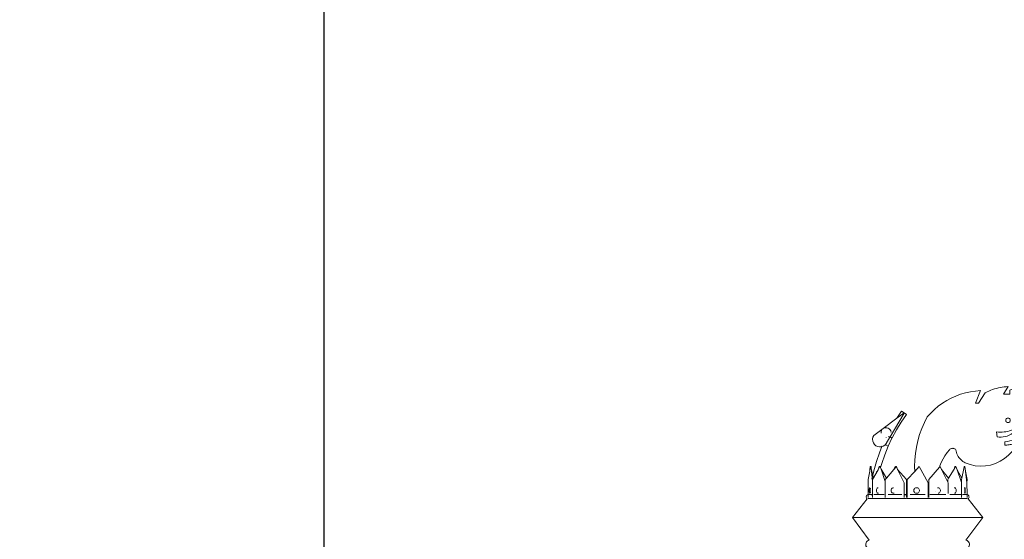
# Model space of a CAD drawing. Units: millimetres. Extents: x 7894 to 8038, y 6851 to 6951.
# Tile 22 of 49: x 7946.6 to 7958.7, y 6910.05 to 6916.43. Entities that reach past the tile are written whole.
import ezdxf

# ---------------------------------------------------------------- set-up
doc = ezdxf.new("R2010")
doc.units = ezdxf.units.MM
doc.layers.add('A-ANNO-DIMS', color=2, linetype='Continuous', lineweight=18)
doc.layers.add('A-FURN-ACCS', color=8, linetype='Continuous', lineweight=13)
doc.styles.get("Standard").update_dxf_attribs({"font": 'arial.ttf'})
doc.dimstyles.new('ISO-25', dxfattribs={"dimtxt": 1, "dimasz": 1, "dimexe": 1.25, "dimexo": 0.625, "dimtad": 1, "dimdec": 0, "dimlunit": 4, "dimtxsty": 'Standard', "dimcen": 2.5, "dimclrt": 1, "dimadec": 0, "dimazin": 0, "dimtfac": 1, "dimtdec": 0, "dimtmove": 0, "dimatfit": 3, "dimfxl": 1, "dimarcsym": 0})

# ---------------------------------------------------------------- blocks, each defined once
blk = doc.blocks.new('DISPLAY-LEAF-FINIAL')
for p, q in [((2.565, 3.508), (2.565, 3.494)), ((2.209, 3.334), (2.276, 3.441)), ((2.276, 3.441), (2.398, 3.441)), ((2.398, 3.441), (2.409, 3.452)), ((2.409, 3.452), (2.421, 3.461)), ((2.421, 3.461), (2.434, 3.47)), ((2.434, 3.47), (2.447, 3.478)), ((2.447, 3.478), (2.461, 3.485)), ((2.461, 3.485), (2.475, 3.491)), ((2.475, 3.491), (2.489, 3.496)), ((2.489, 3.496), (2.504, 3.501)), ((2.504, 3.501), (2.519, 3.504)), ((2.516, 3.389), (2.505, 3.379)), ((2.527, 3.4), (2.516, 3.389)), ((2.536, 3.411), (2.527, 3.4)), ((2.544, 3.424), (2.536, 3.411)), ((2.551, 3.437), (2.544, 3.424)), ((2.556, 3.45), (2.551, 3.437)), ((2.56, 3.465), (2.556, 3.45)), ((2.563, 3.479), (2.56, 3.465)), ((2.565, 3.494), (2.563, 3.479)), ((2.023, 3.221), (2.127, 3.334)), ((2.127, 3.334), (2.209, 3.334)), ((2.493, 3.371), (2.48, 3.364)), ((2.48, 3.364), (2.48, 3.316)), ((2.48, 3.316), (2.533, 3.316)), ((2.505, 3.379), (2.493, 3.371)), ((2.533, 3.316), (2.54, 3.327)), ((2.54, 3.327), (2.549, 3.338)), ((2.549, 3.338), (2.558, 3.347)), ((2.558, 3.347), (2.569, 3.356)), ((2.569, 3.356), (2.58, 3.363)), ((2.58, 3.363), (2.592, 3.37)), ((2.62, 3.27), (2.591, 3.216)), ((2.592, 3.37), (2.604, 3.375)), ((2.604, 3.375), (2.617, 3.379)), ((2.617, 3.379), (2.63, 3.382)), ((2.646, 3.325), (2.62, 3.27)), ((2.63, 3.382), (2.643, 3.383)), ((2.643, 3.383), (2.657, 3.383)), ((2.67, 3.382), (2.646, 3.325)), ((2.657, 3.383), (2.67, 3.382)), ((1.328, 3.133), (1.388, 3.15)), ((1.388, 3.15), (1.449, 3.164)), ((1.449, 3.164), (1.51, 3.173)), ((1.51, 3.173), (1.572, 3.179)), ((1.572, 3.179), (1.511, 3.024)), ((1.55, 3.024), (1.632, 3.152)), ((1.632, 3.152), (1.654, 3.163)), ((1.654, 3.163), (1.676, 3.173)), ((1.676, 3.173), (1.699, 3.182)), ((1.699, 3.182), (1.722, 3.191)), ((1.722, 3.191), (1.745, 3.198)), ((1.745, 3.198), (1.769, 3.205)), ((1.769, 3.205), (1.793, 3.211)), ((1.793, 3.211), (1.817, 3.216)), ((1.817, 3.216), (1.841, 3.22)), ((1.841, 3.22), (1.865, 3.223)), ((1.914, 3.227), (1.854, 3.133)), ((1.865, 3.223), (1.889, 3.226)), ((1.889, 3.226), (1.914, 3.227)), ((1.934, 3.185), (2.023, 3.221)), ((1.934, 3.133), (1.934, 3.185)), ((2.56, 3.163), (2.527, 3.112)), ((2.591, 3.216), (2.56, 3.163)), ((1.105, 3.023), (1.158, 3.056)), ((1.158, 3.056), (1.213, 3.085)), ((1.213, 3.085), (1.27, 3.111)), ((1.27, 3.111), (1.328, 3.133)), ((1.511, 3.024), (1.55, 3.024)), ((1.854, 3.133), (1.934, 3.133)), ((2.491, 3.062), (2.453, 3.014)), ((2.527, 3.112), (2.491, 3.062)), ((0.605, 2.924), (0.547, 2.84)), ((0.634, 2.905), (0.547, 2.84)), ((0.634, 2.905), (0.605, 2.924)), ((0.634, 2.9), (0.634, 2.905)), ((0.663, 2.885), (0.634, 2.905)), ((0.92, 2.857), (0.962, 2.903)), ((0.962, 2.903), (1.007, 2.946)), ((1.007, 2.946), (1.055, 2.986)), ((1.055, 2.986), (1.105, 3.023)), ((2.371, 2.923), (2.327, 2.88)), ((2.413, 2.967), (2.371, 2.923)), ((2.453, 3.014), (2.413, 2.967)), ((0.547, 2.84), (0.379, 2.713)), ((0.634, 2.9), (0.463, 2.609)), ((0.541, 2.696), (0.599, 2.791)), ((0.599, 2.791), (0.663, 2.885)), ((0.884, 2.786), (0.853, 2.713)), ((0.92, 2.857), (0.884, 2.786)), ((1.883, 2.817), (1.885, 2.824)), ((1.883, 2.81), (1.883, 2.817)), ((1.885, 2.803), (1.883, 2.81)), ((1.885, 2.824), (1.889, 2.831)), ((1.888, 2.797), (1.885, 2.803)), ((1.894, 2.791), (1.888, 2.797)), ((1.889, 2.831), (1.894, 2.836)), ((1.894, 2.836), (1.9, 2.839)), ((1.9, 2.788), (1.894, 2.791)), ((1.9, 2.839), (1.907, 2.841)), ((1.907, 2.786), (1.9, 2.788)), ((1.907, 2.841), (1.914, 2.841)), ((1.914, 2.786), (1.907, 2.786)), ((1.914, 2.841), (1.921, 2.839)), ((1.921, 2.788), (1.914, 2.786)), ((1.921, 2.839), (1.928, 2.836)), ((1.928, 2.791), (1.921, 2.788)), ((1.928, 2.836), (1.933, 2.83)), ((1.933, 2.796), (1.928, 2.791)), ((1.933, 2.83), (1.937, 2.824)), ((1.936, 2.803), (1.933, 2.796)), ((1.938, 2.81), (1.936, 2.803)), ((1.937, 2.824), (1.938, 2.817)), ((1.938, 2.817), (1.938, 2.81)), ((2.281, 2.839), (2.233, 2.801)), ((2.233, 2.801), (2.238, 2.792)), ((2.238, 2.792), (2.242, 2.783)), ((2.242, 2.783), (2.245, 2.774)), ((2.327, 2.88), (2.281, 2.839)), ((0.379, 2.713), (0.264, 2.627)), ((0.353, 2.675), (0.358, 2.69)), ((0.353, 2.66), (0.353, 2.675)), ((0.358, 2.69), (0.367, 2.703)), ((0.367, 2.703), (0.379, 2.713)), ((0.379, 2.713), (0.393, 2.72)), ((0.393, 2.72), (0.409, 2.723)), ((0.409, 2.723), (0.425, 2.722)), ((0.425, 2.722), (0.44, 2.718)), ((0.44, 2.718), (0.453, 2.709)), ((0.453, 2.709), (0.464, 2.698)), ((0.464, 2.698), (0.471, 2.684)), ((0.471, 2.684), (0.475, 2.669)), ((0.474, 2.667), (0.475, 2.669)), ((0.474, 2.667), (0.475, 2.666)), ((0.541, 2.696), (0.488, 2.597)), ((0.853, 2.713), (0.826, 2.638)), ((1.793, 2.668), (1.77, 2.67)), ((1.77, 2.67), (1.776, 2.611)), ((1.816, 2.667), (1.793, 2.668)), ((1.84, 2.668), (1.816, 2.667)), ((1.863, 2.67), (1.84, 2.668)), ((1.886, 2.673), (1.863, 2.67)), ((1.909, 2.678), (1.886, 2.673)), ((1.931, 2.684), (1.909, 2.678)), ((1.954, 2.692), (1.931, 2.684)), ((1.975, 2.701), (1.954, 2.692)), ((1.99, 2.673), (1.97, 2.657)), ((1.996, 2.711), (1.975, 2.701)), ((2.007, 2.692), (1.99, 2.673)), ((2.017, 2.722), (1.996, 2.711)), ((2.023, 2.712), (2.007, 2.692)), ((2.036, 2.734), (2.017, 2.722)), ((2.036, 2.734), (2.023, 2.712)), ((2.19, 2.677), (2.164, 2.659)), ((2.216, 2.695), (2.19, 2.677)), ((2.223, 2.702), (2.216, 2.695)), ((2.23, 2.709), (2.223, 2.702)), ((2.235, 2.717), (2.23, 2.709)), ((2.24, 2.726), (2.235, 2.717)), ((2.243, 2.735), (2.24, 2.726)), ((2.245, 2.745), (2.243, 2.735)), ((2.245, 2.774), (2.246, 2.764)), ((2.246, 2.754), (2.245, 2.745)), ((2.246, 2.764), (2.246, 2.754)), ((0.253, 2.607), (0.249, 2.584)), ((0.249, 2.58), (0.249, 2.584)), ((0.249, 2.58), (0.251, 2.557)), ((0.251, 2.557), (0.259, 2.536)), ((0.264, 2.627), (0.253, 2.607)), ((0.353, 2.659), (0.353, 2.66)), ((0.353, 2.657), (0.353, 2.659)), ((0.414, 2.606), (0.413, 2.603)), ((0.461, 2.605), (0.415, 2.527)), ((0.44, 2.496), (0.486, 2.593)), ((0.443, 2.613), (0.446, 2.612)), ((0.451, 2.615), (0.449, 2.616)), ((0.463, 2.609), (0.461, 2.605)), ((0.486, 2.593), (0.461, 2.605)), ((0.463, 2.609), (0.488, 2.597)), ((0.804, 2.562), (0.787, 2.485)), ((0.826, 2.638), (0.804, 2.562)), ((1.801, 2.608), (1.776, 2.611)), ((1.827, 2.607), (1.801, 2.608)), ((1.852, 2.609), (1.827, 2.607)), ((1.878, 2.613), (1.852, 2.609)), ((1.903, 2.554), (1.872, 2.548)), ((1.872, 2.548), (1.872, 2.508)), ((1.902, 2.62), (1.878, 2.613)), ((1.926, 2.63), (1.902, 2.62)), ((1.934, 2.561), (1.903, 2.554)), ((1.949, 2.642), (1.926, 2.63)), ((1.964, 2.569), (1.934, 2.561)), ((1.97, 2.657), (1.949, 2.642)), ((1.994, 2.578), (1.964, 2.569)), ((2.024, 2.588), (1.994, 2.578)), ((2.026, 2.541), (1.997, 2.484)), ((2.013, 2.536), (2.026, 2.541)), ((2.053, 2.6), (2.024, 2.588)), ((2.082, 2.613), (2.053, 2.6)), ((2.11, 2.627), (2.082, 2.613)), ((2.137, 2.643), (2.11, 2.627)), ((2.164, 2.659), (2.137, 2.643)), ((0.259, 2.536), (0.272, 2.517)), ((0.272, 2.517), (0.29, 2.502)), ((0.29, 2.502), (0.311, 2.492)), ((0.311, 2.492), (0.334, 2.488)), ((0.363, 2.491), (0.332, 2.415)), ((0.334, 2.488), (0.358, 2.489)), ((0.358, 2.489), (0.363, 2.491)), ((0.363, 2.491), (0.38, 2.497)), ((0.365, 2.496), (0.363, 2.491)), ((0.38, 2.497), (0.4, 2.51)), ((0.398, 2.513), (0.402, 2.512)), ((0.398, 2.391), (0.44, 2.495)), ((0.403, 2.513), (0.4, 2.514)), ((0.4, 2.51), (0.402, 2.512)), ((0.402, 2.512), (0.403, 2.513)), ((0.402, 2.512), (0.44, 2.495)), ((0.403, 2.513), (0.415, 2.527)), ((0.403, 2.513), (0.44, 2.496)), ((0.409, 2.511), (0.408, 2.509)), ((0.42, 2.535), (0.409, 2.511)), ((0.787, 2.485), (0.774, 2.406)), ((1.193, 2.452), (1.163, 2.417)), ((1.198, 2.457), (1.193, 2.452)), ((1.204, 2.462), (1.198, 2.457)), ((1.211, 2.465), (1.204, 2.462)), ((1.218, 2.467), (1.211, 2.465)), ((1.225, 2.469), (1.218, 2.467)), ((1.232, 2.47), (1.225, 2.469)), ((1.239, 2.469), (1.232, 2.47)), ((1.247, 2.467), (1.239, 2.469)), ((1.254, 2.465), (1.247, 2.467)), ((1.26, 2.462), (1.254, 2.465)), ((1.266, 2.457), (1.26, 2.462)), ((1.271, 2.452), (1.266, 2.457)), ((1.274, 2.435), (1.271, 2.452)), ((1.278, 2.418), (1.274, 2.435)), ((1.872, 2.508), (1.885, 2.509)), ((1.885, 2.509), (1.898, 2.51)), ((1.898, 2.51), (1.911, 2.511)), ((1.911, 2.511), (1.924, 2.513)), ((1.961, 2.432), (1.918, 2.385)), ((1.924, 2.513), (1.937, 2.515)), ((1.937, 2.515), (1.95, 2.518)), ((1.95, 2.518), (1.963, 2.521)), ((1.997, 2.484), (1.961, 2.432)), ((1.963, 2.521), (1.976, 2.524)), ((1.976, 2.524), (1.988, 2.528)), ((1.988, 2.528), (2.001, 2.532)), ((2.001, 2.532), (2.013, 2.536)), ((0.295, 2.306), (0.263, 2.194)), ((0.332, 2.415), (0.295, 2.306)), ((0.361, 2.285), (0.398, 2.391)), ((0.766, 2.327), (0.763, 2.248)), ((0.774, 2.406), (0.766, 2.327)), ((1.092, 2.297), (1.075, 2.254)), ((1.113, 2.339), (1.092, 2.297)), ((1.136, 2.379), (1.113, 2.339)), ((1.163, 2.417), (1.136, 2.379)), ((1.283, 2.402), (1.278, 2.418)), ((1.29, 2.386), (1.283, 2.402)), ((1.298, 2.371), (1.29, 2.386)), ((1.308, 2.357), (1.298, 2.371)), ((1.319, 2.343), (1.308, 2.357)), ((1.331, 2.331), (1.319, 2.343)), ((1.343, 2.319), (1.331, 2.331)), ((1.357, 2.309), (1.343, 2.319)), ((1.372, 2.3), (1.357, 2.309)), ((1.387, 2.292), (1.372, 2.3)), ((1.816, 2.31), (1.759, 2.283)), ((1.87, 2.344), (1.816, 2.31)), ((1.918, 2.385), (1.87, 2.344)), ((0.213, 2.19), (0.195, 2.086)), ((0.213, 2.19), (0.215, 2.201)), ((0.215, 2.201), (0.22, 2.245)), ((0.223, 2.245), (0.215, 2.201)), ((0.223, 2.245), (0.22, 2.245)), ((0.223, 2.245), (0.23, 2.245)), ((0.232, 2.22), (0.23, 2.245)), ((0.232, 2.22), (0.25, 2.138)), ((0.244, 2.11), (0.232, 2.22)), ((0.317, 2.207), (0.248, 2.086)), ((0.263, 2.194), (0.25, 2.138)), ((0.297, 2.185), (0.292, 2.162)), ((0.317, 2.207), (0.33, 2.245)), ((0.338, 2.245), (0.317, 2.207)), ((0.332, 2.245), (0.33, 2.245)), ((0.344, 2.245), (0.338, 2.245)), ((0.347, 2.235), (0.344, 2.245)), ((0.347, 2.235), (0.361, 2.285)), ((0.354, 2.213), (0.347, 2.235)), ((0.354, 2.213), (0.42, 2.104)), ((0.404, 2.061), (0.354, 2.213)), ((0.507, 2.209), (0.42, 2.104)), ((0.507, 2.209), (0.525, 2.245)), ((0.532, 2.239), (0.507, 2.209)), ((0.528, 2.245), (0.525, 2.245)), ((0.528, 2.245), (0.532, 2.239)), ((0.537, 2.245), (0.532, 2.239)), ((0.54, 2.245), (0.537, 2.245)), ((0.556, 2.211), (0.54, 2.245)), ((0.548, 2.22), (0.556, 2.211)), ((0.556, 2.211), (0.663, 2.086)), ((0.636, 2.045), (0.556, 2.211)), ((0.765, 2.186), (0.671, 2.086)), ((0.763, 2.248), (0.765, 2.186)), ((0.821, 2.245), (0.765, 2.186)), ((0.93, 2.045), (0.821, 2.245)), ((1.07, 2.239), (0.939, 2.086)), ((1.07, 2.239), (1.069, 2.235)), ((1.071, 2.24), (1.07, 2.239)), ((1.07, 2.239), (1.071, 2.237)), ((1.075, 2.254), (1.071, 2.24)), ((1.074, 2.245), (1.071, 2.24)), ((1.074, 2.245), (1.078, 2.245)), ((1.095, 2.209), (1.078, 2.245)), ((1.095, 2.209), (1.182, 2.104)), ((1.095, 2.209), (1.171, 2.054)), ((1.248, 2.213), (1.182, 2.104)), ((1.248, 2.213), (1.258, 2.245)), ((1.265, 2.242), (1.248, 2.213)), ((1.258, 2.245), (1.264, 2.245)), ((1.264, 2.245), (1.265, 2.242)), ((1.267, 2.245), (1.265, 2.242)), ((1.267, 2.245), (1.272, 2.245)), ((1.285, 2.207), (1.272, 2.245)), ((1.285, 2.207), (1.344, 2.103)), ((1.285, 2.207), (1.34, 2.048)), ((1.37, 2.22), (1.344, 2.103)), ((1.37, 2.22), (1.372, 2.245)), ((1.375, 2.245), (1.37, 2.22)), ((1.372, 2.245), (1.375, 2.245)), ((1.375, 2.245), (1.382, 2.245)), ((1.382, 2.245), (1.389, 2.19)), ((1.447, 2.27), (1.387, 2.292)), ((1.389, 2.19), (1.408, 2.086)), ((1.407, 2.045), (1.389, 2.19)), ((1.509, 2.256), (1.447, 2.27)), ((1.572, 2.25), (1.509, 2.256)), ((1.635, 2.253), (1.572, 2.25)), ((1.698, 2.264), (1.635, 2.253)), ((1.759, 2.283), (1.698, 2.264)), ((0.195, 2.086), (0.195, 2.048)), ((0.244, 2.11), (0.239, 2.089)), ((0.25, 2.138), (0.244, 2.11)), ((0.248, 2.065), (0.244, 2.11)), ((0.248, 2.086), (0.248, 2.065)), ((0.248, 2.065), (0.248, 1.903)), ((0.25, 2.138), (0.256, 2.115)), ((0.42, 2.104), (0.404, 2.086)), ((0.404, 2.086), (0.404, 2.061)), ((0.404, 2.061), (0.404, 1.901)), ((0.663, 2.086), (0.663, 1.903)), ((0.671, 2.086), (0.671, 1.903)), ((0.939, 2.086), (0.939, 1.934)), ((1.182, 2.104), (1.171, 2.086)), ((1.171, 2.086), (1.171, 2.054)), ((1.344, 2.103), (1.34, 2.086)), ((1.34, 2.086), (1.34, 2.048)), ((1.408, 2.086), (1.407, 2.045)), ((0.195, 2.045), (0.195, 2.048)), ((0.195, 2.045), (0.195, 1.903)), ((0.207, 1.965), (0.208, 1.973)), ((0.207, 1.956), (0.207, 1.965)), ((0.207, 1.947), (0.207, 1.956)), ((0.207, 1.938), (0.207, 1.947)), ((0.208, 1.93), (0.207, 1.938)), ((0.208, 1.973), (0.209, 1.979)), ((0.209, 1.979), (0.211, 1.984)), ((0.21, 1.956), (0.211, 1.965)), ((0.21, 1.947), (0.21, 1.956)), ((0.211, 1.938), (0.21, 1.947)), ((0.211, 1.984), (0.213, 1.986)), ((0.211, 1.965), (0.212, 1.973)), ((0.212, 1.93), (0.211, 1.938)), ((0.212, 1.973), (0.213, 1.979)), ((0.216, 1.986), (0.213, 1.986)), ((0.213, 1.979), (0.214, 1.984)), ((0.216, 1.947), (0.213, 1.924)), ((0.214, 1.984), (0.216, 1.986)), ((0.217, 1.965), (0.216, 1.956)), ((0.216, 1.956), (0.216, 1.947)), ((0.216, 1.947), (0.217, 1.938)), ((0.218, 1.973), (0.217, 1.965)), ((0.218, 1.967), (0.217, 1.965)), ((0.217, 1.938), (0.218, 1.93)), ((0.219, 1.979), (0.218, 1.973)), ((0.218, 1.973), (0.218, 1.967)), ((0.22, 1.981), (0.219, 1.979)), ((0.22, 1.981), (0.219, 1.979)), ((0.221, 1.973), (0.22, 1.965)), ((0.22, 1.965), (0.22, 1.956)), ((0.22, 1.956), (0.22, 1.947)), ((0.22, 1.947), (0.22, 1.938)), ((0.22, 1.938), (0.221, 1.93)), ((0.222, 1.975), (0.221, 1.973)), ((0.295, 1.956), (0.297, 1.965)), ((0.295, 1.947), (0.295, 1.956)), ((0.297, 1.938), (0.295, 1.947)), ((0.297, 1.965), (0.3, 1.973)), ((0.3, 1.93), (0.297, 1.938)), ((0.3, 1.973), (0.304, 1.979)), ((0.304, 1.979), (0.308, 1.984)), ((0.308, 1.984), (0.314, 1.986)), ((0.316, 1.986), (0.314, 1.986)), ((0.476, 1.956), (0.478, 1.965)), ((0.476, 1.947), (0.476, 1.956)), ((0.478, 1.938), (0.476, 1.947)), ((0.478, 1.965), (0.482, 1.973)), ((0.482, 1.93), (0.478, 1.938)), ((0.482, 1.973), (0.488, 1.979)), ((0.488, 1.979), (0.495, 1.984)), ((0.495, 1.984), (0.502, 1.986)), ((0.504, 1.986), (0.502, 1.986)), ((0.636, 2.045), (0.637, 1.903)), ((0.754, 1.956), (0.756, 1.965)), ((0.754, 1.947), (0.754, 1.956)), ((0.756, 1.938), (0.754, 1.947)), ((0.756, 1.965), (0.761, 1.973)), ((0.761, 1.93), (0.756, 1.938)), ((0.761, 1.973), (0.767, 1.979)), ((0.767, 1.979), (0.775, 1.984)), ((0.775, 1.984), (0.784, 1.986)), ((0.784, 1.986), (0.793, 1.986)), ((0.793, 1.986), (0.802, 1.984)), ((0.802, 1.984), (0.81, 1.979)), ((0.81, 1.979), (0.816, 1.973)), ((0.816, 1.973), (0.821, 1.965)), ((0.821, 1.938), (0.816, 1.93)), ((0.821, 1.965), (0.823, 1.956)), ((0.823, 1.947), (0.821, 1.938)), ((0.823, 1.956), (0.823, 1.947)), ((0.93, 2.045), (0.931, 1.934)), ((1.022, 1.935), (1.021, 1.935)), ((1.044, 1.986), (1.046, 1.986)), ((1.046, 1.986), (1.054, 1.986)), ((1.054, 1.986), (1.062, 1.984)), ((1.062, 1.984), (1.069, 1.979)), ((1.069, 1.979), (1.075, 1.973)), ((1.075, 1.973), (1.079, 1.965)), ((1.079, 1.938), (1.075, 1.93)), ((1.079, 1.965), (1.081, 1.956)), ((1.081, 1.947), (1.079, 1.938)), ((1.081, 1.956), (1.081, 1.947)), ((1.176, 2.045), (1.171, 2.054)), ((1.176, 2.045), (1.177, 1.914)), ((1.249, 1.986), (1.251, 1.986)), ((1.251, 1.986), (1.257, 1.986)), ((1.257, 1.986), (1.263, 1.984)), ((1.263, 1.984), (1.268, 1.979)), ((1.268, 1.979), (1.272, 1.973)), ((1.272, 1.973), (1.275, 1.965)), ((1.275, 1.938), (1.272, 1.93)), ((1.275, 1.965), (1.276, 1.956)), ((1.276, 1.947), (1.275, 1.938)), ((1.276, 1.956), (1.276, 1.947)), ((1.341, 2.045), (1.34, 2.048)), ((1.341, 2.045), (1.342, 1.903)), ((1.373, 1.986), (1.376, 1.986)), ((1.376, 1.986), (1.378, 1.984)), ((1.376, 1.986), (1.377, 1.986)), ((1.377, 1.986), (1.379, 1.986)), ((1.378, 1.984), (1.379, 1.979)), ((1.379, 1.986), (1.381, 1.984)), ((1.379, 1.979), (1.381, 1.973)), ((1.381, 1.984), (1.383, 1.979)), ((1.381, 1.973), (1.382, 1.965)), ((1.382, 1.938), (1.381, 1.93)), ((1.382, 1.965), (1.382, 1.956)), ((1.382, 1.956), (1.382, 1.947)), ((1.382, 1.947), (1.382, 1.938)), ((1.383, 1.979), (1.384, 1.973)), ((1.384, 1.973), (1.385, 1.965)), ((1.385, 1.938), (1.384, 1.93)), ((1.385, 1.965), (1.386, 1.956)), ((1.386, 1.947), (1.385, 1.938)), ((1.386, 1.956), (1.386, 1.947)), ((1.407, 2.045), (1.408, 1.903)), ((0, 1.62), (0.181, 1.849)), ((0.17, 1.877), (0.172, 1.885)), ((0.17, 1.87), (0.17, 1.877)), ((0.172, 1.862), (0.17, 1.87)), ((0.172, 1.885), (0.176, 1.892)), ((0.175, 1.855), (0.172, 1.862)), ((0.181, 1.849), (0.175, 1.855)), ((0.176, 1.892), (0.182, 1.898)), ((0.182, 1.898), (0.189, 1.901)), ((0.189, 1.901), (0.195, 1.903)), ((0.195, 1.903), (0.195, 1.901)), ((0.195, 1.903), (0.196, 1.903)), ((0.195, 1.898), (0.195, 1.87)), ((0.195, 1.862), (0.195, 1.855)), ((0.195, 1.855), (0.195, 1.855)), ((0.205, 1.855), (0.195, 1.855)), ((0.196, 1.903), (0.198, 1.903)), ((0.196, 1.903), (0.197, 1.903)), ((0.237, 1.903), (0.198, 1.903)), ((0.205, 1.855), (0.205, 1.851)), ((0.248, 1.855), (0.205, 1.855)), ((0.205, 1.851), (0.205, 1.849)), ((0.209, 1.924), (0.208, 1.93)), ((0.211, 1.919), (0.209, 1.924)), ((0.213, 1.917), (0.211, 1.919)), ((0.213, 1.924), (0.212, 1.93)), ((0.214, 1.919), (0.213, 1.924)), ((0.214, 1.917), (0.213, 1.917)), ((0.216, 1.917), (0.214, 1.919)), ((0.216, 1.917), (0.214, 1.917)), ((0.218, 1.917), (0.216, 1.917)), ((0.218, 1.93), (0.219, 1.924)), ((0.219, 1.924), (0.22, 1.921)), ((0.221, 1.93), (0.222, 1.928)), ((0.24, 1.855), (0.24, 1.849)), ((0.248, 1.903), (0.244, 1.903)), ((0.245, 1.898), (0.244, 1.886)), ((0.248, 1.897), (0.244, 1.897)), ((0.248, 1.925), (0.246, 1.901)), ((0.248, 1.903), (0.248, 1.901)), ((0.248, 1.898), (0.248, 1.897)), ((0.248, 1.897), (0.248, 1.87)), ((0.248, 1.862), (0.248, 1.855)), ((0.248, 1.855), (0.276, 1.855)), ((0.391, 1.903), (0.265, 1.903)), ((0.275, 1.849), (0.276, 1.855)), ((0.276, 1.855), (0.405, 1.855)), ((0.303, 1.924), (0.3, 1.93)), ((0.308, 1.919), (0.303, 1.924)), ((0.313, 1.917), (0.308, 1.919)), ((0.319, 1.917), (0.313, 1.917)), ((0.322, 1.917), (0.319, 1.917)), ((0.404, 1.898), (0.404, 1.87)), ((0.404, 1.862), (0.405, 1.855)), ((0.405, 1.855), (0.637, 1.855)), ((0.439, 1.903), (0.607, 1.903)), ((0.488, 1.924), (0.482, 1.93)), ((0.495, 1.919), (0.488, 1.924)), ((0.502, 1.917), (0.495, 1.919)), ((0.51, 1.917), (0.502, 1.917)), ((0.512, 1.917), (0.51, 1.917)), ((0.637, 1.903), (0.634, 1.903)), ((0.637, 1.897), (0.634, 1.897)), ((0.637, 1.903), (0.637, 1.901)), ((0.663, 1.903), (0.637, 1.903)), ((0.637, 1.898), (0.637, 1.897)), ((0.637, 1.897), (0.637, 1.87)), ((0.663, 1.897), (0.637, 1.897)), ((0.637, 1.862), (0.637, 1.855)), ((0.663, 1.855), (0.637, 1.855)), ((0.663, 1.903), (0.671, 1.903)), ((0.663, 1.903), (0.663, 1.901)), ((0.663, 1.898), (0.663, 1.897)), ((0.663, 1.897), (0.663, 1.87)), ((0.671, 1.897), (0.663, 1.897)), ((0.663, 1.862), (0.663, 1.855)), ((0.671, 1.903), (0.671, 1.901)), ((0.671, 1.898), (0.671, 1.897)), ((0.671, 1.897), (0.671, 1.87)), ((0.671, 1.862), (0.671, 1.855)), ((0.671, 1.855), (0.932, 1.855)), ((0.708, 1.903), (0.894, 1.903)), ((0.767, 1.924), (0.761, 1.93)), ((0.775, 1.919), (0.767, 1.924)), ((0.784, 1.917), (0.775, 1.919)), ((0.793, 1.917), (0.784, 1.917)), ((0.802, 1.919), (0.793, 1.917)), ((0.81, 1.924), (0.802, 1.919)), ((0.816, 1.93), (0.81, 1.924)), ((0.939, 1.934), (0.931, 1.934)), ((0.931, 1.934), (0.931, 1.903)), ((0.931, 1.903), (0.931, 1.901)), ((0.939, 1.903), (0.931, 1.903)), ((0.931, 1.898), (0.931, 1.897)), ((0.931, 1.897), (0.932, 1.87)), ((0.939, 1.897), (0.931, 1.897)), ((0.932, 1.862), (0.932, 1.855)), ((0.939, 1.855), (0.932, 1.855)), ((0.942, 1.934), (0.939, 1.934)), ((0.939, 1.934), (0.939, 1.903)), ((0.942, 1.903), (0.939, 1.903)), ((0.939, 1.903), (0.939, 1.901)), ((0.939, 1.898), (0.939, 1.897)), ((0.942, 1.897), (0.939, 1.897)), ((0.939, 1.897), (0.939, 1.87)), ((0.939, 1.862), (0.939, 1.855)), ((1.342, 1.855), (0.939, 1.855)), ((0.953, 1.903), (1.146, 1.903)), ((1.052, 1.917), (1.054, 1.917)), ((1.062, 1.919), (1.054, 1.917)), ((1.069, 1.924), (1.062, 1.919)), ((1.075, 1.93), (1.069, 1.924)), ((1.33, 1.903), (1.197, 1.903)), ((1.254, 1.917), (1.257, 1.917)), ((1.263, 1.919), (1.257, 1.917)), ((1.268, 1.924), (1.263, 1.919)), ((1.272, 1.93), (1.268, 1.924)), ((1.347, 1.903), (1.342, 1.903)), ((1.342, 1.903), (1.342, 1.901)), ((1.342, 1.898), (1.342, 1.897)), ((1.347, 1.897), (1.342, 1.897)), ((1.342, 1.897), (1.342, 1.87)), ((1.342, 1.862), (1.342, 1.855)), ((1.408, 1.855), (1.342, 1.855)), ((1.356, 1.903), (1.4, 1.903)), ((1.378, 1.919), (1.375, 1.917)), ((1.375, 1.917), (1.379, 1.917)), ((1.379, 1.924), (1.378, 1.919)), ((1.381, 1.93), (1.379, 1.924)), ((1.381, 1.919), (1.379, 1.917)), ((1.383, 1.924), (1.381, 1.919)), ((1.384, 1.93), (1.383, 1.924)), ((1.408, 1.903), (1.413, 1.901)), ((1.408, 1.903), (1.408, 1.901)), ((1.408, 1.898), (1.408, 1.87)), ((1.408, 1.862), (1.408, 1.855)), ((1.413, 1.901), (1.42, 1.898)), ((1.42, 1.898), (1.426, 1.892)), ((1.427, 1.855), (1.421, 1.849)), ((1.421, 1.849), (1.602, 1.62)), ((1.426, 1.892), (1.43, 1.885)), ((1.431, 1.862), (1.427, 1.855)), ((1.43, 1.885), (1.432, 1.877)), ((1.433, 1.87), (1.431, 1.862)), ((1.432, 1.877), (1.433, 1.87)), ((0.207, 1.343), (0, 1.62)), ((1.602, 1.62), (0, 1.62)), ((1.602, 1.62), (1.395, 1.343)), ((0.174, 1.321), (0.183, 1.331)), ((0.183, 1.331), (0.195, 1.338)), ((0.195, 1.338), (0.207, 1.343)), ((1.395, 1.343), (1.408, 1.338)), ((1.408, 1.338), (1.419, 1.331)), ((1.419, 1.331), (1.428, 1.321)), ((0.164, 1.297), (0.168, 1.31)), ((0.164, 1.283), (0.164, 1.297)), ((0.167, 1.27), (0.164, 1.283)), ((0.173, 1.258), (0.167, 1.27)), ((0.168, 1.31), (0.174, 1.321)), ((0.171, 0.955), (0.191, 1.234)), ((0.182, 1.248), (0.173, 1.258)), ((0.193, 1.24), (0.182, 1.248)), ((0.219, 1.234), (0.191, 1.234)), ((0.206, 1.236), (0.193, 1.24)), ((0.196, 0.954), (0.311, 1.21)), ((0.219, 1.234), (0.206, 1.236)), ((0.219, 1.234), (0.297, 1.234)), ((0.297, 1.234), (0.302, 1.234)), ((0.303, 1.232), (0.297, 1.234)), ((0.303, 1.232), (0.302, 1.234)), ((0.302, 1.234), (0.594, 1.234)), ((0.311, 1.21), (0.303, 1.232)), ((0.324, 1.172), (0.311, 1.21)), ((0.434, 0.975), (0.609, 1.228)), ((0.594, 1.234), (0.617, 1.234)), ((0.609, 1.228), (0.594, 1.234)), ((0.617, 1.228), (0.617, 1.234)), ((0.952, 1.234), (0.617, 1.234)), ((0.632, 1.205), (0.617, 1.228)), ((0.86, 1.041), (0.977, 1.215)), ((0.981, 1.234), (0.952, 1.234)), ((0.977, 1.215), (0.974, 1.218)), ((0.99, 1.195), (0.977, 1.215)), ((0.981, 1.234), (0.982, 1.234)), ((0.982, 1.234), (0.983, 1.234)), ((1.284, 1.234), (0.983, 1.234)), ((1.177, 0.964), (1.275, 1.212)), ((1.275, 1.212), (1.283, 1.232)), ((1.285, 1.19), (1.275, 1.212)), ((1.283, 1.232), (1.29, 1.234)), ((1.283, 1.232), (1.284, 1.234)), ((1.284, 1.234), (1.29, 1.234)), ((1.29, 1.234), (1.383, 1.234)), ((1.397, 1.236), (1.383, 1.234)), ((1.41, 1.234), (1.383, 1.234)), ((1.409, 1.24), (1.397, 1.236)), ((1.42, 1.248), (1.409, 1.24)), ((1.411, 1.234), (1.41, 1.234)), ((1.411, 1.232), (1.411, 1.234)), ((1.435, 0.955), (1.411, 1.232)), ((1.42, 0.955), (1.411, 1.232)), ((1.429, 1.258), (1.42, 1.248)), ((1.428, 1.321), (1.434, 1.31)), ((1.435, 1.27), (1.429, 1.258)), ((1.434, 1.31), (1.438, 1.297)), ((1.438, 1.283), (1.435, 1.27)), ((1.438, 1.297), (1.438, 1.283)), ((0.194, 1.111), (0.196, 1.124)), ((0.195, 1.101), (0.194, 1.111)), ((0.196, 1.094), (0.195, 1.101)), ((0.196, 1.124), (0.198, 1.137)), ((0.199, 1.09), (0.196, 1.094)), ((0.198, 1.137), (0.202, 1.152)), ((0.203, 1.089), (0.199, 1.09)), ((0.202, 1.152), (0.206, 1.165)), ((0.204, 1.088), (0.203, 1.089)), ((0.206, 1.165), (0.212, 1.177)), ((0.211, 1.096), (0.213, 1.092)), ((0.212, 1.177), (0.217, 1.187)), ((0.213, 1.092), (0.214, 1.092)), ((0.214, 1.1), (0.214, 1.098)), ((0.215, 0.949), (0.324, 1.172)), ((0.217, 1.187), (0.223, 1.193)), ((0.223, 1.193), (0.228, 1.197)), ((0.228, 1.197), (0.232, 1.196)), ((0.232, 1.195), (0.232, 1.196)), ((0.232, 1.195), (0.237, 1.195)), ((0.402, 0.955), (0.324, 1.172)), ((0.387, 1.137), (0.389, 1.152)), ((0.387, 1.124), (0.387, 1.137)), ((0.391, 1.111), (0.387, 1.124)), ((0.389, 1.152), (0.395, 1.165)), ((0.397, 1.101), (0.391, 1.111)), ((0.395, 1.165), (0.403, 1.177)), ((0.406, 1.094), (0.397, 1.101)), ((0.403, 1.177), (0.413, 1.187)), ((0.409, 1.092), (0.406, 1.094)), ((0.413, 1.187), (0.424, 1.193)), ((0.424, 1.193), (0.436, 1.197)), ((0.436, 1.197), (0.448, 1.196)), ((0.448, 1.196), (0.458, 1.192)), ((0.455, 0.949), (0.632, 1.205)), ((0.458, 1.192), (0.461, 1.191)), ((0.742, 1.037), (0.632, 1.205)), ((0.747, 1.137), (0.748, 1.152)), ((0.747, 1.136), (0.747, 1.137)), ((0.748, 1.152), (0.752, 1.165)), ((0.752, 1.165), (0.76, 1.177)), ((0.76, 1.177), (0.77, 1.187)), ((0.77, 1.187), (0.783, 1.193)), ((0.783, 1.193), (0.797, 1.197)), ((0.797, 1.197), (0.812, 1.196)), ((0.812, 1.196), (0.826, 1.192)), ((0.826, 1.192), (0.838, 1.185)), ((0.838, 1.185), (0.848, 1.175)), ((0.848, 1.175), (0.855, 1.162)), ((0.855, 1.162), (0.859, 1.148)), ((0.859, 1.147), (0.859, 1.148)), ((0.86, 0.992), (0.99, 1.195)), ((1.16, 0.949), (0.99, 1.195)), ((1.124, 1.192), (1.126, 1.193)), ((1.126, 1.193), (1.127, 1.193)), ((1.127, 1.193), (1.138, 1.197)), ((1.138, 1.197), (1.15, 1.196)), ((1.15, 1.196), (1.162, 1.192)), ((1.162, 1.192), (1.174, 1.185)), ((1.174, 1.092), (1.172, 1.091)), ((1.174, 1.185), (1.184, 1.175)), ((1.174, 1.092), (1.175, 1.092)), ((1.185, 1.099), (1.175, 1.092)), ((1.184, 1.175), (1.191, 1.162)), ((1.192, 1.109), (1.185, 1.099)), ((1.191, 1.162), (1.196, 1.148)), ((1.196, 1.121), (1.192, 1.109)), ((1.196, 1.148), (1.198, 1.134)), ((1.198, 1.134), (1.196, 1.121)), ((1.202, 0.955), (1.285, 1.19)), ((1.398, 0.949), (1.285, 1.19)), ((1.359, 1.195), (1.364, 1.197)), ((1.359, 1.195), (1.362, 1.195)), ((1.364, 1.197), (1.369, 1.196)), ((1.369, 1.196), (1.374, 1.192)), ((1.374, 1.192), (1.38, 1.185)), ((1.38, 1.185), (1.386, 1.175)), ((1.386, 1.175), (1.392, 1.162)), ((1.392, 1.089), (1.39, 1.088)), ((1.39, 1.088), (1.395, 1.089)), ((1.392, 1.162), (1.396, 1.148)), ((1.399, 1.092), (1.395, 1.089)), ((1.396, 1.148), (1.4, 1.134)), ((1.401, 1.099), (1.399, 1.092)), ((1.4, 1.134), (1.402, 1.121)), ((1.402, 1.109), (1.401, 1.099)), ((1.402, 1.121), (1.402, 1.109)), ((0.416, 0.949), (0.434, 0.975)), ((0.442, 0.955), (0.434, 0.975)), ((0.742, 0), (0.742, 1.037)), ((0.799, 0.949), (0.742, 1.037)), ((0.799, 0.949), (0.816, 0.974)), ((0.816, 0.974), (0.814, 0.977)), ((0.816, 0.974), (0.86, 1.041)), ((0.816, 0.973), (0.816, 0.974)), ((0.843, 0.965), (0.86, 0.992)), ((0.86, 1.041), (0.86, 1.047)), ((0.86, 0.992), (0.86, 1.041)), ((0.86, 0), (0.86, 0.992)), ((0.194, 0.949), (0.171, 0.955)), ((0.194, 0.949), (0.196, 0.954)), ((0.215, 0.949), (0.196, 0.954)), ((0.416, 0.949), (0.402, 0.955)), ((0.455, 0.949), (0.442, 0.955)), ((1.16, 0.949), (1.173, 0.955)), ((1.173, 0.955), (1.177, 0.964)), ((1.187, 0.949), (1.177, 0.964)), ((1.187, 0.949), (1.202, 0.955)), ((1.398, 0.949), (1.41, 0.953)), ((1.41, 0.953), (1.42, 0.955)), ((1.412, 0.949), (1.41, 0.953)), ((1.412, 0.949), (1.435, 0.955))]:
    blk.add_line(p, q)
blk = doc.blocks.new('*D23')
at = {"layer": 'A-ANNO-DIMS', "color": 0, "lineweight": -2, "transparency": 16777216}
for p, q in [((7940.089, 6907.098), (7940.089, 6947.793)), ((7971.936, 6928.989), (7971.936, 6947.793)), ((7941.089, 6946.543), (7970.936, 6946.543))]:
    blk.add_line(p, q, dxfattribs=at)
at = {"layer": 'A-ANNO-DIMS', "color": 0, "transparency": 16777216}
for points in [[(7941.089, 6946.709), (7941.089, 6946.376), (7940.089, 6946.543)], [(7970.936, 6946.709), (7970.936, 6946.376), (7971.936, 6946.543)]]:
    blk.add_solid(points, dxfattribs=at)
at = {"layer": 'Defpoints', "color": 0, "transparency": 16777216}
for p in [(7971.936, 6946.543), (7971.936, 6928.364), (7940.089, 6906.473)]:
    blk.add_point(p, dxfattribs=at)
at = {"layer": 'A-ANNO-DIMS', "color": 1, "transparency": 16777216, "insert": (7956.012, 6947.678), "char_height": 1, "attachment_point": 5}
blk.add_mtext('2\'-8"', dxfattribs=at)
blk = doc.blocks.new('*D24')
at = {"layer": 'A-ANNO-DIMS', "color": 0, "lineweight": -2, "transparency": 16777216}
for p, q in [((7953.341, 6944.606), (7936.902, 6944.606)), ((7938.152, 6907.473), (7938.152, 6943.606)), ((7939.464, 6906.473), (7936.902, 6906.473))]:
    blk.add_line(p, q, dxfattribs=at)
at = {"layer": 'A-ANNO-DIMS', "color": 0, "transparency": 16777216}
for points in [[(7937.986, 6943.606), (7938.319, 6943.606), (7938.152, 6944.606)], [(7937.986, 6907.473), (7938.319, 6907.473), (7938.152, 6906.473)]]:
    blk.add_solid(points, dxfattribs=at)
at = {"layer": 'Defpoints', "color": 0, "transparency": 16777216}
for p in [(7938.152, 6944.606), (7953.966, 6944.606), (7940.089, 6906.473)]:
    blk.add_point(p, dxfattribs=at)
at = {"layer": 'A-ANNO-DIMS', "color": 1, "transparency": 16777216, "insert": (7937.016, 6925.539), "char_height": 1, "attachment_point": 5, "rotation": 90}
blk.add_mtext('3\'-2"', dxfattribs=at)
blk = doc.blocks.new('*D26')
at = {"layer": 'A-ANNO-DIMS', "color": 0, "lineweight": -2, "transparency": 16777216}
for p, q in [((7950.965, 6918.72), (7975.227, 6918.72)), ((7973.977, 6917.72), (7973.977, 6907.473)), ((7964.966, 6906.473), (7975.227, 6906.473))]:
    blk.add_line(p, q, dxfattribs=at)
at = {"layer": 'A-ANNO-DIMS', "color": 0, "transparency": 16777216}
for points in [[(7973.811, 6917.72), (7974.144, 6917.72), (7973.977, 6918.72)], [(7973.811, 6907.473), (7974.144, 6907.473), (7973.977, 6906.473)]]:
    blk.add_solid(points, dxfattribs=at)
at = {"layer": 'Defpoints', "color": 0, "transparency": 16777216}
for p in [(7950.34, 6918.72), (7964.341, 6906.473), (7973.977, 6906.473)]:
    blk.add_point(p, dxfattribs=at)
at = {"layer": 'A-ANNO-DIMS', "color": 1, "transparency": 16777216, "insert": (7972.842, 6912.597), "char_height": 1, "attachment_point": 5, "rotation": 90}
blk.add_mtext('1\'-0"', dxfattribs=at)
blk = doc.blocks.new('*D29')
at = {"layer": 'A-ANNO-DIMS', "color": 0, "lineweight": -2, "transparency": 16777216}
for p, q in [((7940.435, 6923.814), (7940.435, 6903.287)), ((7943.737, 6918.095), (7943.737, 6903.287)), ((7941.435, 6904.537), (7942.737, 6904.537)), ((7943.737, 6904.537), (7950.975, 6904.537))]:
    blk.add_line(p, q, dxfattribs=at)
at = {"layer": 'A-ANNO-DIMS', "color": 0, "transparency": 16777216}
for points in [[(7941.435, 6904.703), (7941.435, 6904.37), (7940.435, 6904.537)], [(7942.737, 6904.703), (7942.737, 6904.37), (7943.737, 6904.537)]]:
    blk.add_solid(points, dxfattribs=at)
at = {"layer": 'Defpoints', "color": 0, "transparency": 16777216}
for p in [(7940.435, 6924.439), (7943.737, 6918.72), (7943.737, 6904.537)]:
    blk.add_point(p, dxfattribs=at)
at = {"layer": 'A-ANNO-DIMS', "color": 1, "transparency": 16777216, "insert": (7947.856, 6905.679), "char_height": 1, "attachment_point": 5}
blk.add_mtext('0\'-3 1/2"', dxfattribs=at)
blk = doc.blocks.new('*D32')
at = {"layer": 'A-ANNO-DIMS', "color": 0, "lineweight": -2, "transparency": 16777216}
for p, q in [((7943.737, 6918.095), (7943.737, 6903.287)), ((7950.34, 6918.095), (7950.34, 6903.287)), ((7944.737, 6904.537), (7949.34, 6904.537))]:
    blk.add_line(p, q, dxfattribs=at)
at = {"layer": 'A-ANNO-DIMS', "color": 0, "transparency": 16777216}
for points in [[(7944.737, 6904.703), (7944.737, 6904.37), (7943.737, 6904.537)], [(7949.34, 6904.703), (7949.34, 6904.37), (7950.34, 6904.537)]]:
    blk.add_solid(points, dxfattribs=at)
at = {"layer": 'Defpoints', "color": 0, "transparency": 16777216}
for p in [(7943.737, 6918.72), (7950.34, 6918.72), (7950.34, 6904.537)]:
    blk.add_point(p, dxfattribs=at)
at = {"layer": 'A-ANNO-DIMS', "color": 1, "transparency": 16777216, "insert": (7947.038, 6905.679), "char_height": 1, "attachment_point": 5}
blk.add_mtext('0\'-6 1/2"', dxfattribs=at)
blk = doc.blocks.new('*D33')
at = {"layer": 'A-ANNO-DIMS', "color": 0, "lineweight": -2, "transparency": 16777216}
for p, q in [((7940.435, 6923.814), (7940.435, 6903.287)), ((7940.089, 6905.848), (7940.089, 6903.287)), ((7939.089, 6904.537), (7938.089, 6904.537)), ((7940.089, 6904.537), (7940.435, 6904.537)), ((7941.435, 6904.537), (7948.673, 6904.537))]:
    blk.add_line(p, q, dxfattribs=at)
at = {"layer": 'A-ANNO-DIMS', "color": 0, "transparency": 16777216}
for points in [[(7939.089, 6904.703), (7939.089, 6904.37), (7940.089, 6904.537)], [(7941.435, 6904.703), (7941.435, 6904.37), (7940.435, 6904.537)]]:
    blk.add_solid(points, dxfattribs=at)
at = {"layer": 'Defpoints', "color": 0, "transparency": 16777216}
for p in [(7940.435, 6924.439), (7940.089, 6906.473), (7940.435, 6904.537)]:
    blk.add_point(p, dxfattribs=at)
at = {"layer": 'A-ANNO-DIMS', "color": 1, "transparency": 16777216, "insert": (7945.554, 6905.679), "char_height": 1, "attachment_point": 5}
blk.add_mtext('0\'-0 1/2"', dxfattribs=at)

msp = doc.modelspace()

# ---------------------------------------------------------------- block references
at = {"layer": 'A-FURN-ACCS'}
msp.add_blockref('DISPLAY-LEAF-FINIAL', (7956.83, 6908.701), dxfattribs=at)

# ---------------------------------------------------------------- dimensions: what is measured, and where the dimension line sits
at = {"layer": 'A-ANNO-DIMS'}
for base, p1, p2, picture, middle in [((7971.936, 6946.543), (7940.089, 6906.473), (7971.936, 6928.364), '*D23', (7956.012, 6947.678)), ((7940.435, 6904.537), (7940.089, 6906.473), (7940.435, 6924.439), '*D33', (7945.554, 6905.679)), ((7943.737, 6904.537), (7940.435, 6924.439), (7943.737, 6918.72), '*D29', (7947.856, 6905.679)), ((7950.34, 6904.537), (7943.737, 6918.72), (7950.34, 6918.72), '*D32', (7947.038, 6905.679))]:
    dim = msp.add_linear_dim(base=base, p1=p1, p2=p2, dimstyle='ISO-25', override={"dimdec": 1, "dimlfac": 1, "dimrnd": 0, "dimzin": 1, "dimdsep": 46, "dimlunit": 4, "dimfrac": 2}, dxfattribs=at)
    dim.commit()
    dim.dimension.update_dxf_attribs({"geometry": picture, "text_midpoint": middle})
for base, p1, p2, picture, middle in [((7938.152, 6944.606), (7940.089, 6906.473), (7953.966, 6944.606), '*D24', (7937.016, 6925.539)), ((7973.977, 6906.473), (7950.34, 6918.72), (7964.341, 6906.473), '*D26', (7972.842, 6912.597))]:
    dim = msp.add_linear_dim(base=base, p1=p1, p2=p2, angle=90, dimstyle='ISO-25', override={"dimdec": 1, "dimlfac": 1, "dimrnd": 0, "dimzin": 1, "dimdsep": 46, "dimlunit": 4, "dimfrac": 2}, dxfattribs=at)
    dim.commit()
    dim.dimension.update_dxf_attribs({"geometry": picture, "text_midpoint": middle})

doc.saveas('drawing.dxf')
